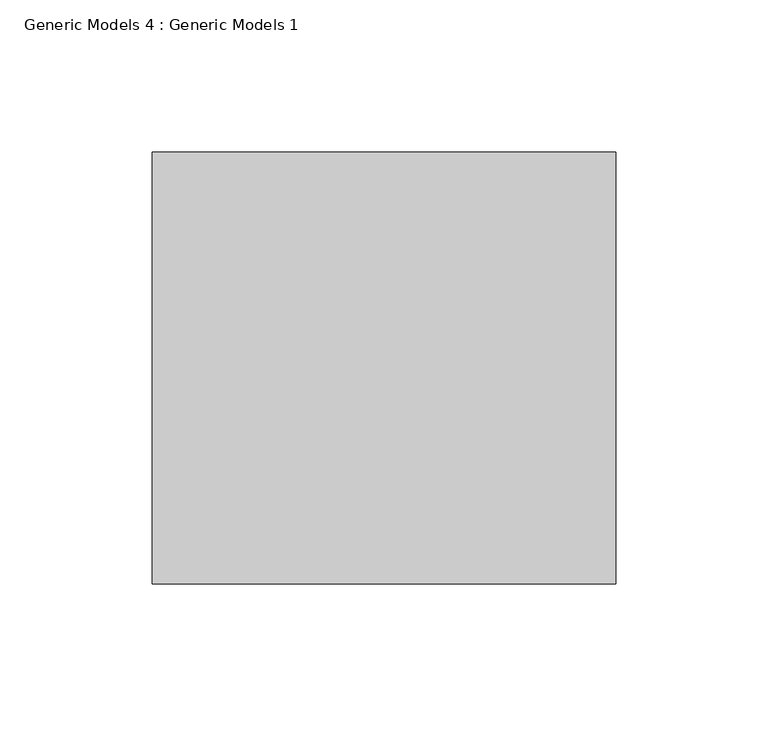
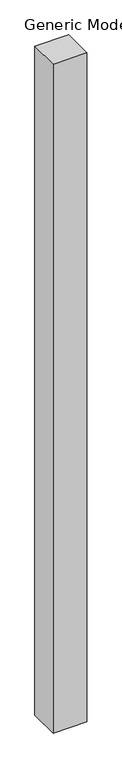
"""IFC4 building model written with IfcOpenShell, lengths in millimetres: proxy geometry, Generic Models 4 : Generic Models 1."""

from ifc_helpers import new_model, si_unit, origin, origin_with_axes, place, context, project, spatial, polyline, outline, extrude, source, transform, mapped, element, save


def generic_models_4_generic_models_1_fab6a1cf(model_context):
    return source(origin(), model_context, "Body", "SweptSolid", [
        extrude(outline(polyline([(-10384.7326527, -5471.7273102), (-10232.3326527, -5471.7273102), (-10232.3326527, -5613.7098142), (-10384.7326527, -5613.7098142), (-10384.7326527, -5471.7273102)])), origin_with_axes(), (0.0, 0.0, 1.0), 3200.4),
    ])


if __name__ == "__main__":
    model = new_model("IFC4")
    model_context = context("Model", 3, world=origin())
    ifc_project = project(units=[si_unit("LENGTHUNIT", "METRE", prefix="MILLI")], contexts=[model_context])
    site = spatial("IfcSite", under=ifc_project)
    building = spatial("IfcBuilding", under=site)
    placement = place(None, origin())
    generic_models_4_generic_models_1_shape = generic_models_4_generic_models_1_fab6a1cf(model_context)
    element("IfcBuildingElementProxy", 1, Name="Generic Models 4 : Generic Models 1", ObjectType="Generic Models 4 : Generic Models 1", at=placement, inside=building, context=model_context, shape_type="MappedRepresentation", body=[
        mapped(generic_models_4_generic_models_1_shape, transform((0.0, 0.0, 0.0), x_axis=(1.0, 0.0, 0.0), y_axis=(0.0, 1.0, 0.0), z_axis=(0.0, 0.0, 1.0))),
    ])
    save(model, "model.ifc")
